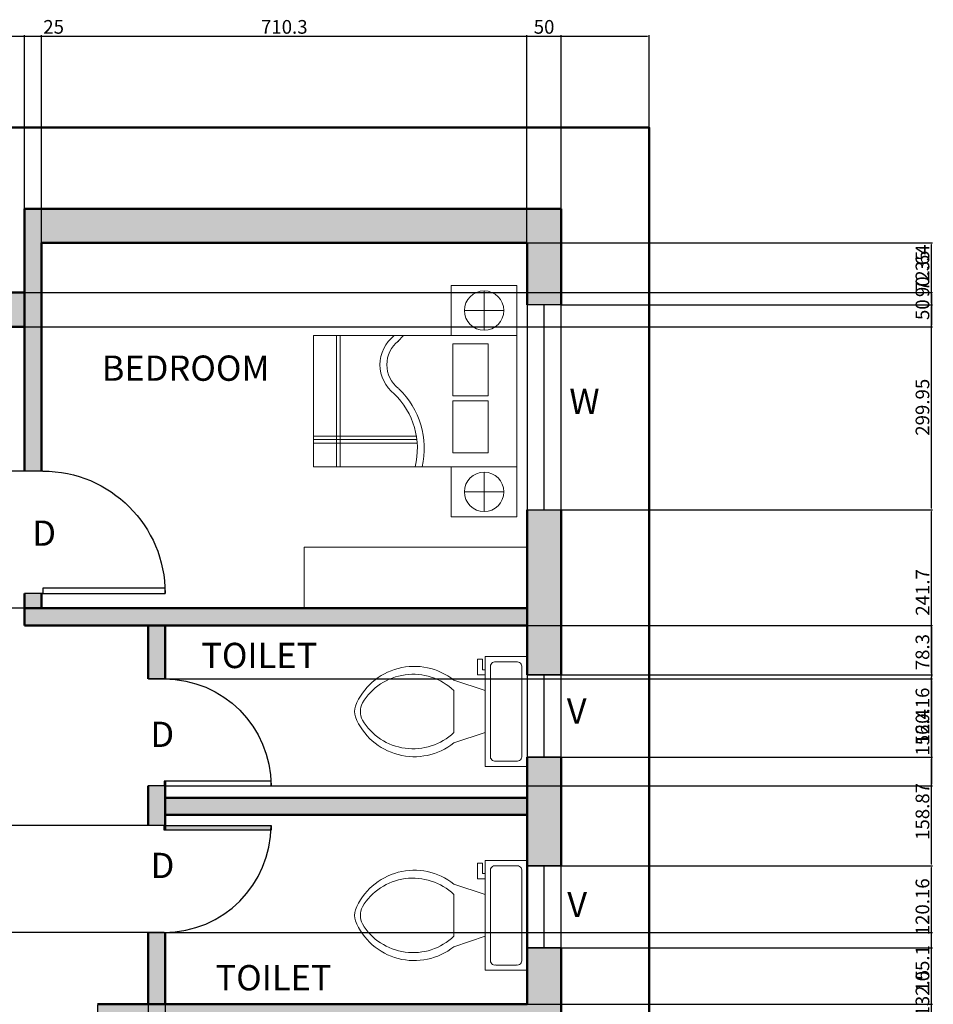
# Model space of a CAD drawing. Units: millimetres. Extents: x 1898 to 8115, y 727 to 4291.
# Tile 7 of 7: x 6778 to 8115, y 2277 to 3717. Entities that reach past the tile are written whole.
import ezdxf

# ---------------------------------------------------------------- set-up
doc = ezdxf.new("R2010")
doc.units = ezdxf.units.MM
for name, color, linetype, lineweight in [('A-ANNO-DIMS', 2, 'Continuous', 18), ('A-ANNO-TEXT', 7, 'Continuous', 25), ('A-AREA-IDEN', 3, 'Continuous', 25), ('A-DOOR', 3, 'Continuous', 25), ('A-FLOR-FIXT', 9, 'Continuous', 18), ('A-FURN', 8, 'Continuous', 18), ('A-GLAZ', 4, 'Continuous', 25), ('A-WALL', 7, 'Continuous', 50), ('A-WALL-PATT', 8, 'Continuous', 13)]:
    doc.layers.add(name, color=color, linetype=linetype, lineweight=lineweight)
doc.styles.get("Standard").update_dxf_attribs({"font": 'arial.ttf'})
doc.dimstyles.new('ISO-25', dxfattribs={"dimtxt": 20, "dimasz": 2.5, "dimexe": 1.25, "dimexo": 0.625, "dimtad": 1, "dimtxsty": 'Standard', "dimcen": 2.5, "dimadec": 0, "dimazin": 0, "dimtfac": 1, "dimtmove": 0, "dimatfit": 3, "dimfxl": 1, "dimarcsym": 0})

# ---------------------------------------------------------------- blocks, each defined once
blk = doc.blocks.new('*U43')
for p, q in [((0, 0), (0, -6)), ((40, 0), (40, -6))]:
    blk.add_line(p, q)
blk.add_lwpolyline([(0, 0), (0, 40), (1.75, 40), (1.75, 0)], close=True)
blk.add_arc((0, 0), 40, 0, 90)
blk = doc.blocks.new('*U45')
for p, q in [((9.5, -6), (9.5, -2)), ((-10, -8.5), (-8, -8.5)), ((-10, -9.5), (-10, -8.5)), ((-8, -8.5), (-8, -8)), ((-7, -8), (-7, -9.5)), ((-4, -8), (-6, -14)), ((4, -8), (6, -14)), ((-7, -9.5), (-10, -9.5)), ((4, -14), (-4, -14))]:
    blk.add_line(p, q)
blk.add_lwpolyline([(10.5, -8), (10.5, 0), (-10.5, 0), (-10.5, -8)], close=True)
for points in [[(8.5, -1), (-8.5, -1)], [(-9.5, -2), (-9.5, -6)], [(-8.5, -7), (8.5, -7)]]:
    blk.add_lwpolyline(points)
for centre, radius, start, end in [((-8.62, -1.88), 0.884, 81.8699, 188.1301), ((8.62, -1.88), 0.884, 351.8699, 98.1301), ((-8.62, -6.12), 0.884, 171.8699, 278.1301), ((8.62, -6.12), 0.884, 261.8699, 8.1301), ((3.52, -21.58), 12.17, 141.4691, 247.9714), ((4.2, -21.82), 11.33, 136.3677, 238.9468), ((-3.52, -21.58), 12.17, 292.0284, 38.5307), ((-4.2, -21.82), 11.33, 301.053, 43.6321), ((0, -27.88), 4, 245.7318, 294.2682), ((0, -29), 4, 254.8605, 285.1395)]:
    blk.add_arc(centre, radius, start, end)
blk = doc.blocks.new('*D57')
at = {"layer": 'A-ANNO-DIMS', "color": 0, "lineweight": -2, "transparency": 16777216}
for p, q in [((5348.6, 3560.4), (5348.6, 3694.5)), ((5351.1, 3693.2), (7696.3, 3693.2)), ((7698.8, 3560.4), (7698.8, 3694.5))]:
    blk.add_line(p, q, dxfattribs=at)
at = {"layer": 'A-ANNO-DIMS', "color": 0, "transparency": 16777216}
for points in [[(5351.1, 3693.7), (5351.1, 3692.8), (5348.6, 3693.2)], [(7696.3, 3693.7), (7696.3, 3692.8), (7698.8, 3693.2)]]:
    blk.add_solid(points, dxfattribs=at)
at = {"layer": 'Defpoints', "color": 0, "transparency": 16777216}
for p in [(7698.8, 3693.2), (5348.6, 3559.7), (7698.8, 3559.7)]:
    blk.add_point(p, dxfattribs=at)
at = {"layer": 'A-ANNO-DIMS', "color": 0, "transparency": 16777216, "insert": (6523.7, 3704.1), "char_height": 20, "attachment_point": 5}
blk.add_mtext('2350', dxfattribs=at)
blk = doc.blocks.new('*D58')
at = {"layer": 'A-ANNO-DIMS', "color": 0, "lineweight": -2, "transparency": 16777216}
for p, q in [((5461.6, 3441.3), (5461.6, 3694.5)), ((5464.1, 3693.2), (7567.7, 3693.2)), ((7570.2, 3441.3), (7570.2, 3694.5))]:
    blk.add_line(p, q, dxfattribs=at)
at = {"layer": 'A-ANNO-DIMS', "color": 0, "transparency": 16777216}
for points in [[(5464.1, 3693.7), (5464.1, 3692.8), (5461.6, 3693.2)], [(7567.7, 3693.7), (7567.7, 3692.8), (7570.2, 3693.2)]]:
    blk.add_solid(points, dxfattribs=at)
at = {"layer": 'Defpoints', "color": 0, "transparency": 16777216}
for p in [(7570.2, 3693.2), (5461.6, 3440.7), (7570.2, 3440.7)]:
    blk.add_point(p, dxfattribs=at)
at = {"layer": 'A-ANNO-DIMS', "color": 0, "transparency": 16777216, "insert": (6515.9, 3704.1), "char_height": 20, "attachment_point": 5}
blk.add_mtext('2108.6', dxfattribs=at)
blk = doc.blocks.new('*D66')
at = {"layer": 'A-ANNO-DIMS', "color": 0, "lineweight": -2, "transparency": 16777216}
for p, q in [((6201.7, 3318.6), (6201.7, 3694.5)), ((6204.2, 3693.2), (6782.4, 3693.2)), ((6784.9, 3318.6), (6784.9, 3694.5))]:
    blk.add_line(p, q, dxfattribs=at)
at = {"layer": 'A-ANNO-DIMS', "color": 0, "transparency": 16777216}
for points in [[(6204.2, 3693.7), (6204.2, 3692.8), (6201.7, 3693.2)], [(6782.4, 3693.7), (6782.4, 3692.8), (6784.9, 3693.2)]]:
    blk.add_solid(points, dxfattribs=at)
at = {"layer": 'Defpoints', "color": 0, "transparency": 16777216}
for p in [(6784.9, 3693.2), (6201.7, 3318), (6784.9, 3318)]:
    blk.add_point(p, dxfattribs=at)
at = {"layer": 'A-ANNO-DIMS', "color": 0, "transparency": 16777216, "insert": (6493.3, 3704.1), "char_height": 20, "attachment_point": 5}
blk.add_mtext('583.2', dxfattribs=at)
blk = doc.blocks.new('*D67')
at = {"layer": 'A-ANNO-DIMS', "color": 0, "lineweight": -2, "transparency": 16777216}
for p, q in [((6784.9, 3318.6), (6784.9, 3694.5)), ((6787.4, 3693.2), (6807.4, 3693.2)), ((6809.9, 3391.3), (6809.9, 3694.5)), ((6809.9, 3693.2), (6842.8, 3693.2))]:
    blk.add_line(p, q, dxfattribs=at)
at = {"layer": 'A-ANNO-DIMS', "color": 0, "transparency": 16777216}
for points in [[(6787.4, 3693.7), (6787.4, 3692.8), (6784.9, 3693.2)], [(6807.4, 3693.7), (6807.4, 3692.8), (6809.9, 3693.2)]]:
    blk.add_solid(points, dxfattribs=at)
at = {"layer": 'Defpoints', "color": 0, "transparency": 16777216}
for p in [(6809.9, 3693.2), (6809.9, 3390.7), (6784.9, 3318)]:
    blk.add_point(p, dxfattribs=at)
at = {"layer": 'A-ANNO-DIMS', "color": 0, "transparency": 16777216, "insert": (6827.6, 3704.1), "char_height": 20, "attachment_point": 5}
blk.add_mtext('25', dxfattribs=at)
blk = doc.blocks.new('*D68')
at = {"layer": 'A-ANNO-DIMS', "color": 0, "lineweight": -2, "transparency": 16777216}
for p, q in [((6809.9, 3391.3), (6809.9, 3694.5)), ((6812.4, 3693.2), (7517.7, 3693.2)), ((7520.2, 3391.3), (7520.2, 3694.5))]:
    blk.add_line(p, q, dxfattribs=at)
at = {"layer": 'A-ANNO-DIMS', "color": 0, "transparency": 16777216}
for points in [[(6812.4, 3693.7), (6812.4, 3692.8), (6809.9, 3693.2)], [(7517.7, 3693.7), (7517.7, 3692.8), (7520.2, 3693.2)]]:
    blk.add_solid(points, dxfattribs=at)
at = {"layer": 'Defpoints', "color": 0, "transparency": 16777216}
for p in [(7520.2, 3693.2), (6809.9, 3390.7), (7520.2, 3390.7)]:
    blk.add_point(p, dxfattribs=at)
at = {"layer": 'A-ANNO-DIMS', "color": 0, "transparency": 16777216, "insert": (7165.1, 3704.1), "char_height": 20, "attachment_point": 5}
blk.add_mtext('710.3', dxfattribs=at)
blk = doc.blocks.new('*D69')
at = {"layer": 'A-ANNO-DIMS', "color": 0, "lineweight": -2, "transparency": 16777216}
for p, q in [((7520.2, 3391.3), (7520.2, 3694.5)), ((7522.7, 3693.2), (7567.7, 3693.2)), ((7570.2, 3300.9), (7570.2, 3694.5))]:
    blk.add_line(p, q, dxfattribs=at)
at = {"layer": 'A-ANNO-DIMS', "color": 0, "transparency": 16777216}
for points in [[(7522.7, 3693.7), (7522.7, 3692.8), (7520.2, 3693.2)], [(7567.7, 3693.7), (7567.7, 3692.8), (7570.2, 3693.2)]]:
    blk.add_solid(points, dxfattribs=at)
at = {"layer": 'Defpoints', "color": 0, "transparency": 16777216}
for p in [(7570.2, 3693.2), (7520.2, 3390.7), (7570.2, 3300.3)]:
    blk.add_point(p, dxfattribs=at)
at = {"layer": 'A-ANNO-DIMS', "color": 0, "transparency": 16777216, "insert": (7545.2, 3704.1), "char_height": 20, "attachment_point": 5}
blk.add_mtext('50', dxfattribs=at)
blk = doc.blocks.new('*D94')
at = {"layer": 'A-ANNO-DIMS', "color": 0, "lineweight": -2, "transparency": 16777216}
for p, q in [((7570.8, 2359.5), (8113.5, 2359.5)), ((8112.2, 2229.5), (8112.2, 2357)), ((7570.8, 2227), (8113.5, 2227))]:
    blk.add_line(p, q, dxfattribs=at)
at = {"layer": 'A-ANNO-DIMS', "color": 0, "transparency": 16777216}
for points in [[(8111.8, 2357), (8112.7, 2357), (8112.2, 2359.5)], [(8111.8, 2229.5), (8112.7, 2229.5), (8112.2, 2227)]]:
    blk.add_solid(points, dxfattribs=at)
at = {"layer": 'Defpoints', "color": 0, "transparency": 16777216}
for p in [(7570.2, 2359.5), (8112.2, 2359.5), (7570.2, 2227)]:
    blk.add_point(p, dxfattribs=at)
at = {"layer": 'A-ANNO-DIMS', "color": 0, "transparency": 16777216, "insert": (8101.4, 2293.2), "char_height": 20, "attachment_point": 5, "rotation": 90}
blk.add_mtext('132.5', dxfattribs=at)
blk = doc.blocks.new('*D95')
at = {"layer": 'A-ANNO-DIMS', "color": 0, "lineweight": -2, "transparency": 16777216}
for p, q in [((7570.8, 2479.6), (8113.5, 2479.6)), ((8112.2, 2362), (8112.2, 2477.1)), ((7570.8, 2359.5), (8113.5, 2359.5))]:
    blk.add_line(p, q, dxfattribs=at)
at = {"layer": 'A-ANNO-DIMS', "color": 0, "transparency": 16777216}
for points in [[(8111.8, 2477.1), (8112.7, 2477.1), (8112.2, 2479.6)], [(8111.8, 2362), (8112.7, 2362), (8112.2, 2359.5)]]:
    blk.add_solid(points, dxfattribs=at)
at = {"layer": 'Defpoints', "color": 0, "transparency": 16777216}
for p in [(7570.2, 2479.6), (8112.2, 2479.6), (7570.2, 2359.5)]:
    blk.add_point(p, dxfattribs=at)
at = {"layer": 'A-ANNO-DIMS', "color": 0, "transparency": 16777216, "insert": (8101.4, 2419.6), "char_height": 20, "attachment_point": 5, "rotation": 90}
blk.add_mtext('120.16', dxfattribs=at)
blk = doc.blocks.new('*D96')
at = {"layer": 'A-ANNO-DIMS', "color": 0, "lineweight": -2, "transparency": 16777216}
for p, q in [((7570.8, 2638.5), (8113.5, 2638.5)), ((8112.2, 2482.1), (8112.2, 2636)), ((7570.8, 2479.6), (8113.5, 2479.6))]:
    blk.add_line(p, q, dxfattribs=at)
at = {"layer": 'A-ANNO-DIMS', "color": 0, "transparency": 16777216}
for points in [[(8111.8, 2636), (8112.7, 2636), (8112.2, 2638.5)], [(8111.8, 2482.1), (8112.7, 2482.1), (8112.2, 2479.6)]]:
    blk.add_solid(points, dxfattribs=at)
at = {"layer": 'Defpoints', "color": 0, "transparency": 16777216}
for p in [(7570.2, 2638.5), (8112.2, 2638.5), (7570.2, 2479.6)]:
    blk.add_point(p, dxfattribs=at)
at = {"layer": 'A-ANNO-DIMS', "color": 0, "transparency": 16777216, "insert": (8101.4, 2559.1), "char_height": 20, "attachment_point": 5, "rotation": 90}
blk.add_mtext('158.87', dxfattribs=at)
blk = doc.blocks.new('*D97')
at = {"layer": 'A-ANNO-DIMS', "color": 0, "lineweight": -2, "transparency": 16777216}
for p, q in [((7570.8, 2758.7), (8113.5, 2758.7)), ((8112.2, 2641), (8112.2, 2756.2)), ((7570.8, 2638.5), (8113.5, 2638.5))]:
    blk.add_line(p, q, dxfattribs=at)
at = {"layer": 'A-ANNO-DIMS', "color": 0, "transparency": 16777216}
for points in [[(8111.8, 2756.2), (8112.7, 2756.2), (8112.2, 2758.7)], [(8111.8, 2641), (8112.7, 2641), (8112.2, 2638.5)]]:
    blk.add_solid(points, dxfattribs=at)
at = {"layer": 'Defpoints', "color": 0, "transparency": 16777216}
for p in [(7570.2, 2758.7), (8112.2, 2758.7), (7570.2, 2638.5)]:
    blk.add_point(p, dxfattribs=at)
at = {"layer": 'A-ANNO-DIMS', "color": 0, "transparency": 16777216, "insert": (8101.4, 2698.6), "char_height": 20, "attachment_point": 5, "rotation": 90}
blk.add_mtext('120.16', dxfattribs=at)
blk = doc.blocks.new('*D98')
at = {"layer": 'A-ANNO-DIMS', "color": 0, "lineweight": -2, "transparency": 16777216}
for p, q in [((7570.8, 3000.4), (8113.5, 3000.4)), ((8112.2, 2761.2), (8112.2, 2997.9)), ((7570.8, 2758.7), (8113.5, 2758.7))]:
    blk.add_line(p, q, dxfattribs=at)
at = {"layer": 'A-ANNO-DIMS', "color": 0, "transparency": 16777216}
for points in [[(8111.8, 2997.9), (8112.7, 2997.9), (8112.2, 3000.4)], [(8111.8, 2761.2), (8112.7, 2761.2), (8112.2, 2758.7)]]:
    blk.add_solid(points, dxfattribs=at)
at = {"layer": 'Defpoints', "color": 0, "transparency": 16777216}
for p in [(7570.2, 3000.4), (8112.2, 3000.4), (7570.2, 2758.7)]:
    blk.add_point(p, dxfattribs=at)
at = {"layer": 'A-ANNO-DIMS', "color": 0, "transparency": 16777216, "insert": (8101.6, 2879.5), "char_height": 20, "attachment_point": 5, "rotation": 90}
blk.add_mtext('241.7', dxfattribs=at)
blk = doc.blocks.new('*D99')
at = {"layer": 'A-ANNO-DIMS', "color": 0, "lineweight": -2, "transparency": 16777216}
for p, q in [((7570.8, 3300.3), (8113.5, 3300.3)), ((8112.2, 3002.9), (8112.2, 3297.8)), ((7570.8, 3000.4), (8113.5, 3000.4))]:
    blk.add_line(p, q, dxfattribs=at)
at = {"layer": 'A-ANNO-DIMS', "color": 0, "transparency": 16777216}
for points in [[(8111.8, 3297.8), (8112.7, 3297.8), (8112.2, 3300.3)], [(8111.8, 3002.9), (8112.7, 3002.9), (8112.2, 3000.4)]]:
    blk.add_solid(points, dxfattribs=at)
at = {"layer": 'Defpoints', "color": 0, "transparency": 16777216}
for p in [(7570.2, 3300.3), (8112.2, 3300.3), (7570.2, 3000.4)]:
    blk.add_point(p, dxfattribs=at)
at = {"layer": 'A-ANNO-DIMS', "color": 0, "transparency": 16777216, "insert": (8101.4, 3150.3), "char_height": 20, "attachment_point": 5, "rotation": 90}
blk.add_mtext('299.95', dxfattribs=at)
blk = doc.blocks.new('*D100')
at = {"layer": 'A-ANNO-DIMS', "color": 0, "lineweight": -2, "transparency": 16777216}
for p, q in [((7520.8, 3390.7), (8113.5, 3390.7)), ((8112.2, 3302.8), (8112.2, 3388.2)), ((7570.8, 3300.3), (8113.5, 3300.3))]:
    blk.add_line(p, q, dxfattribs=at)
at = {"layer": 'A-ANNO-DIMS', "color": 0, "transparency": 16777216}
for points in [[(8111.8, 3388.2), (8112.7, 3388.2), (8112.2, 3390.7)], [(8111.8, 3302.8), (8112.7, 3302.8), (8112.2, 3300.3)]]:
    blk.add_solid(points, dxfattribs=at)
at = {"layer": 'Defpoints', "color": 0, "transparency": 16777216}
for p in [(7520.2, 3390.7), (8112.2, 3390.7), (7570.2, 3300.3)]:
    blk.add_point(p, dxfattribs=at)
at = {"layer": 'A-ANNO-DIMS', "color": 0, "transparency": 16777216, "insert": (8101.4, 3345.5), "char_height": 20, "attachment_point": 5, "rotation": 90}
blk.add_mtext('90.35', dxfattribs=at)
blk = doc.blocks.new('*D101')
at = {"layer": 'A-ANNO-DIMS', "color": 0, "lineweight": -2, "transparency": 16777216}
for p, q in [((6810.5, 3390.7), (8113.5, 3390.7)), ((8112.2, 3320.5), (8112.2, 3388.2)), ((6785.5, 3318), (8113.5, 3318))]:
    blk.add_line(p, q, dxfattribs=at)
at = {"layer": 'A-ANNO-DIMS', "color": 0, "transparency": 16777216}
for points in [[(8111.8, 3388.2), (8112.7, 3388.2), (8112.2, 3390.7)], [(8111.8, 3320.5), (8112.7, 3320.5), (8112.2, 3318)]]:
    blk.add_solid(points, dxfattribs=at)
at = {"layer": 'Defpoints', "color": 0, "transparency": 16777216}
for p in [(6809.9, 3390.7), (8112.2, 3390.7), (6784.9, 3318)]:
    blk.add_point(p, dxfattribs=at)
at = {"layer": 'A-ANNO-DIMS', "color": 0, "transparency": 16777216, "insert": (8101.4, 3354.3), "char_height": 20, "attachment_point": 5, "rotation": 90}
blk.add_mtext('72.64', dxfattribs=at)
blk = doc.blocks.new('*D102')
at = {"layer": 'A-ANNO-DIMS', "color": 0, "lineweight": -2, "transparency": 16777216}
for p, q in [((6785.5, 3318), (8113.5, 3318)), ((8112.2, 3315.5), (8112.2, 3270.5)), ((6785.5, 3268), (8113.5, 3268))]:
    blk.add_line(p, q, dxfattribs=at)
at = {"layer": 'A-ANNO-DIMS', "color": 0, "transparency": 16777216}
for points in [[(8111.8, 3315.5), (8112.7, 3315.5), (8112.2, 3318)], [(8111.8, 3270.5), (8112.7, 3270.5), (8112.2, 3268)]]:
    blk.add_solid(points, dxfattribs=at)
at = {"layer": 'Defpoints', "color": 0, "transparency": 16777216}
for p in [(6784.9, 3318), (6784.9, 3268), (8112.2, 3268)]:
    blk.add_point(p, dxfattribs=at)
at = {"layer": 'A-ANNO-DIMS', "color": 0, "transparency": 16777216, "insert": (8101.4, 3293), "char_height": 20, "attachment_point": 5, "rotation": 90}
blk.add_mtext('50', dxfattribs=at)
blk = doc.blocks.new('*D108')
at = {"layer": 'A-ANNO-DIMS', "color": 0, "lineweight": -2, "transparency": 16777216}
for p, q in [((6891.7, 2276.3), (6891.7, 1080.3)), ((6965.8, 2276.3), (6965.8, 1080.3)), ((6894.2, 1081.6), (6963.3, 1081.6))]:
    blk.add_line(p, q, dxfattribs=at)
at = {"layer": 'A-ANNO-DIMS', "color": 0, "transparency": 16777216}
for points in [[(6894.2, 1082), (6894.2, 1081.2), (6891.7, 1081.6)], [(6963.3, 1082), (6963.3, 1081.2), (6965.8, 1081.6)]]:
    blk.add_solid(points, dxfattribs=at)
at = {"layer": 'Defpoints', "color": 0, "transparency": 16777216}
for p in [(6891.7, 2277), (6965.8, 2277), (6965.8, 1081.6)]:
    blk.add_point(p, dxfattribs=at)
at = {"layer": 'A-ANNO-DIMS', "color": 0, "transparency": 16777216, "insert": (6928.8, 1092.4), "char_height": 20, "attachment_point": 5}
blk.add_mtext('74.15', dxfattribs=at)
blk = doc.blocks.new('*D109')
at = {"layer": 'A-ANNO-DIMS', "color": 0, "lineweight": -2, "transparency": 16777216}
for p, q in [((6965.8, 2276.3), (6965.8, 1080.3)), ((6990.8, 2276.3), (6990.8, 1080.3)), ((6968.3, 1081.6), (6988.3, 1081.6)), ((6990.8, 1081.6), (7023.7, 1081.6))]:
    blk.add_line(p, q, dxfattribs=at)
at = {"layer": 'A-ANNO-DIMS', "color": 0, "transparency": 16777216}
for points in [[(6968.3, 1082), (6968.3, 1081.2), (6965.8, 1081.6)], [(6988.3, 1082), (6988.3, 1081.2), (6990.8, 1081.6)]]:
    blk.add_solid(points, dxfattribs=at)
at = {"layer": 'Defpoints', "color": 0, "transparency": 16777216}
for p in [(6965.8, 2277), (6990.8, 2277), (6990.8, 1081.6)]:
    blk.add_point(p, dxfattribs=at)
at = {"layer": 'A-ANNO-DIMS', "color": 0, "transparency": 16777216, "insert": (7008.5, 1092.4), "char_height": 20, "attachment_point": 5}
blk.add_mtext('25', dxfattribs=at)
blk = doc.blocks.new('*D110')
at = {"layer": 'A-ANNO-DIMS', "color": 0, "lineweight": -2, "transparency": 16777216}
for p, q in [((6809.3, 3057), (5213.8, 3057)), ((5215.1, 2858.8), (5215.1, 3054.5)), ((6809.3, 2856.3), (5213.8, 2856.3))]:
    blk.add_line(p, q, dxfattribs=at)
at = {"layer": 'A-ANNO-DIMS', "color": 0, "transparency": 16777216}
for points in [[(5214.6, 3054.5), (5215.5, 3054.5), (5215.1, 3057)], [(5214.6, 2858.8), (5215.5, 2858.8), (5215.1, 2856.3)]]:
    blk.add_solid(points, dxfattribs=at)
at = {"layer": 'Defpoints', "color": 0, "transparency": 16777216}
for p in [(5215.1, 3057), (6809.9, 3057), (6809.9, 2856.3)]:
    blk.add_point(p, dxfattribs=at)
at = {"layer": 'A-ANNO-DIMS', "color": 0, "transparency": 16777216, "insert": (5204.2, 2956.6), "char_height": 20, "attachment_point": 5, "rotation": 90}
blk.add_mtext('200.72', dxfattribs=at)
blk = doc.blocks.new('*D111')
at = {"layer": 'A-ANNO-DIMS', "color": 0, "lineweight": -2, "transparency": 16777216}
for p, q in [((6966.5, 2831.3), (8113.5, 2831.3)), ((8112.2, 2828.8), (8112.2, 2755.5)), ((6966.5, 2753), (8113.5, 2753))]:
    blk.add_line(p, q, dxfattribs=at)
at = {"layer": 'A-ANNO-DIMS', "color": 0, "transparency": 16777216}
for points in [[(8111.8, 2828.8), (8112.7, 2828.8), (8112.2, 2831.3)], [(8111.8, 2755.5), (8112.7, 2755.5), (8112.2, 2753)]]:
    blk.add_solid(points, dxfattribs=at)
at = {"layer": 'Defpoints', "color": 0, "transparency": 16777216}
for p in [(6965.8, 2831.3), (6965.8, 2753), (8112.2, 2753)]:
    blk.add_point(p, dxfattribs=at)
at = {"layer": 'A-ANNO-DIMS', "color": 0, "transparency": 16777216, "insert": (8101.4, 2792.1), "char_height": 20, "attachment_point": 5, "rotation": 90}
blk.add_mtext('78.3', dxfattribs=at)
blk = doc.blocks.new('*D112')
at = {"layer": 'A-ANNO-DIMS', "color": 0, "lineweight": -2, "transparency": 16777216}
for p, q in [((6991.5, 2753), (8113.5, 2753)), ((8112.2, 2750.5), (8112.2, 2599.1)), ((6989.9, 2596.6), (8113.5, 2596.6))]:
    blk.add_line(p, q, dxfattribs=at)
at = {"layer": 'A-ANNO-DIMS', "color": 0, "transparency": 16777216}
for points in [[(8111.8, 2750.5), (8112.7, 2750.5), (8112.2, 2753)], [(8111.8, 2599.1), (8112.7, 2599.1), (8112.2, 2596.6)]]:
    blk.add_solid(points, dxfattribs=at)
at = {"layer": 'Defpoints', "color": 0, "transparency": 16777216}
for p in [(6990.8, 2753), (6989.3, 2596.6), (8112.2, 2596.6)]:
    blk.add_point(p, dxfattribs=at)
at = {"layer": 'A-ANNO-DIMS', "color": 0, "transparency": 16777216, "insert": (8101.4, 2674.8), "char_height": 20, "attachment_point": 5, "rotation": 90}
blk.add_mtext('156.4', dxfattribs=at)
blk = doc.blocks.new('*D113')
at = {"layer": 'A-ANNO-DIMS', "color": 0, "lineweight": -2, "transparency": 16777216}
for p, q in [((6965.2, 2538.5), (5213.8, 2538.5)), ((5215.1, 2536), (5215.1, 2384.6)), ((6965.2, 2382.1), (5213.8, 2382.1))]:
    blk.add_line(p, q, dxfattribs=at)
at = {"layer": 'A-ANNO-DIMS', "color": 0, "transparency": 16777216}
for points in [[(5214.6, 2536), (5215.5, 2536), (5215.1, 2538.5)], [(5214.6, 2384.6), (5215.5, 2384.6), (5215.1, 2382.1)]]:
    blk.add_solid(points, dxfattribs=at)
at = {"layer": 'Defpoints', "color": 0, "transparency": 16777216}
for p in [(6965.8, 2538.5), (5215.1, 2382.1), (6965.8, 2382.1)]:
    blk.add_point(p, dxfattribs=at)
at = {"layer": 'A-ANNO-DIMS', "color": 0, "transparency": 16777216, "insert": (5204.2, 2460.3), "char_height": 20, "attachment_point": 5, "rotation": 90}
blk.add_mtext('156.42', dxfattribs=at)
blk = doc.blocks.new('*D114')
at = {"layer": 'A-ANNO-DIMS', "color": 0, "lineweight": -2, "transparency": 16777216}
for p, q in [((6966.5, 2382.1), (8113.5, 2382.1)), ((8112.2, 2279.5), (8112.2, 2379.6)), ((6966.5, 2277), (8113.5, 2277))]:
    blk.add_line(p, q, dxfattribs=at)
at = {"layer": 'A-ANNO-DIMS', "color": 0, "transparency": 16777216}
for points in [[(8111.8, 2379.6), (8112.7, 2379.6), (8112.2, 2382.1)], [(8111.8, 2279.5), (8112.7, 2279.5), (8112.2, 2277)]]:
    blk.add_solid(points, dxfattribs=at)
at = {"layer": 'Defpoints', "color": 0, "transparency": 16777216}
for p in [(6965.8, 2382.1), (8112.2, 2382.1), (6965.8, 2277)]:
    blk.add_point(p, dxfattribs=at)
at = {"layer": 'A-ANNO-DIMS', "color": 0, "transparency": 16777216, "insert": (8101.4, 2329.5), "char_height": 20, "attachment_point": 5, "rotation": 90}
blk.add_mtext('105.1', dxfattribs=at)

msp = doc.modelspace()

# ---------------------------------------------------------------- hatches: boundary and pattern name
at = {"layer": 'A-WALL-PATT'}
h = msp.add_hatch(color=256, dxfattribs=at)
h.dxf.hatch_style = 1
h.paths.add_polyline_path([(6201.726, 3440.661), (5461.585, 3440.661), (5461.585, 3265.221), (5511.585, 3265.221), (5511.585, 3390.661), (6176.726, 3390.661), (6176.726, 2856.284), (6201.726, 2856.284)])
h.paths.add_polyline_path([(6784.895, 3318.017), (6201.726, 3318.017), (6201.726, 3268.017), (6784.895, 3268.017)])
h.paths.add_polyline_path([(7570.217, 3440.661), (6784.895, 3440.661), (6784.895, 3057.009), (6809.895, 3057.009), (6809.895, 3390.661), (7520.217, 3390.661), (7520.217, 3300.311), (7570.217, 3300.311)])
h.paths.add_polyline_path([(7570.217, 3000.359), (7520.217, 3000.359), (7520.217, 2758.681), (7570.217, 2758.681)])
h.paths.add_polyline_path([(7520.217, 2856.284), (7194.283, 2856.284), (6784.895, 2856.284), (6784.895, 2831.284), (7520.217, 2831.284)])
h.paths.add_polyline_path([(6809.895, 2878.069), (6784.895, 2878.069), (6784.895, 2856.284), (6809.895, 2856.284)])
h.paths.add_polyline_path([(6201.726, 2856.284), (6176.726, 2856.284), (6161.551, 2856.284), (6161.551, 2831.284), (6201.726, 2831.284)])
h.paths.add_polyline_path([(5905.861, 2856.284), (5511.585, 2856.284), (5511.585, 2831.284), (5905.861, 2831.284)])
h.paths.add_polyline_path([(5511.585, 2965.269), (5461.585, 2965.269), (5461.585, 2698.678), (5511.585, 2698.678)])
h.paths.add_polyline_path([(5511.585, 2398.725), (5461.585, 2398.725), (5461.585, 2088.028), (5511.585, 2088.028)])
h.paths.add_polyline_path([(5989.6, 2238.621), (5989.6, 2276.975), (5511.585, 2276.975), (5511.585, 2226.975), (5989.865, 2226.975, -0.01139164)])
h.paths.add_polyline_path([(6636.013, 2276.975), (6245.29, 2276.975), (6245.29, 2238.621), (6245.29, 2226.975), (6636.013, 2226.975), (6636.013, 2238.621)])
h.paths.add_polyline_path([(7570.217, 2359.481), (7520.217, 2359.481), (7520.217, 2326.802), (7520.217, 2276.975), (6891.704, 2276.975), (6891.704, 2238.621, -0.01139164), (6891.439, 2226.975), (7570.217, 2226.975)])
h.paths.add_polyline_path([(7145.586, 2531.644), (6989.313, 2531.644), (6989.313, 2538.488), (7145.735, 2538.488), (7145.735, 2531.644), (7145.586, 2531.644, -0.39860379), (6990.849, 2382.073), (6990.849, 2276.975), (6965.849, 2276.975), (6965.849, 2382.065), (6989.313, 2382.065, 0.40145271)])
h.paths.add_polyline_path([(6990.849, 2596.561), (6989.313, 2596.561), (6965.849, 2596.561), (6965.849, 2538.488), (6990.849, 2538.488)])
h.paths.add_polyline_path([(6990.849, 2831.284), (6965.849, 2831.284), (6965.849, 2752.984), (6990.849, 2752.984)])
h.paths.add_polyline_path([(7570.217, 2638.517), (7520.217, 2638.517), (7520.217, 2625.002), (7520.217, 2479.644), (7570.217, 2479.644)])
h.paths.add_polyline_path([(7520.217, 2579.13), (6990.849, 2579.13), (6990.849, 2554.13), (7520.217, 2554.13)])

# ---------------------------------------------------------------- linework, layer by layer
at = {"layer": 'A-FURN'}
for p, q in [((7457.414, 3262.89), (7457.414, 3320.499)), ((7486.219, 3291.695), (7428.61, 3291.695)), ((7241.696, 3063.119), (7241.696, 3255.036)), ((7246.696, 3063.119), (7246.696, 3255.036)), ((7331.427, 3246.671), (7339.669, 3255.036)), ((7359.058, 3107.895), (7207.596, 3107.895)), ((7359.058, 3102.895), (7207.596, 3102.895)), ((7359.058, 3097.895), (7207.596, 3097.895)), ((7457.414, 2997.657), (7457.414, 3055.266)), ((7486.219, 3026.461), (7428.61, 3026.461))]:
    msp.add_line(p, q, dxfattribs=at)
for points in [[(7505.435, 3255.036), (7409.393, 3255.036), (7409.393, 3328.353), (7505.435, 3328.353)], [(7505.435, 3255.036), (7207.596, 3255.036), (7207.596, 3063.119), (7505.435, 3063.119)], [(7463.586, 3167.185), (7411.519, 3167.185), (7411.519, 3243.164), (7463.586, 3243.164)], [(7463.586, 3083.676), (7411.519, 3083.676), (7411.519, 3159.655), (7463.586, 3159.655)], [(7505.435, 2989.803), (7409.393, 2989.803), (7409.393, 3063.119), (7505.435, 3063.119)], [(7194.283, 2856.284), (7520.217, 2856.284), (7520.217, 2945.821), (7194.283, 2945.821)]]:
    msp.add_lwpolyline(points, close=True, dxfattribs=at)
for centre in [(7457.414, 3291.695), (7457.414, 3026.461)]:
    msp.add_circle(centre, 28.804, dxfattribs=at)
for centre, radius, start, end in [((7359.1, 3212.48), 53.987, 127.974461, 232.025539), ((7359.1, 3212.48), 43.987, 127.974461, 232.025539), ((7248.669, 3089.981), 111.142, 346.014043, 45.994834), ((7248.669, 3089.981), 121.142, 347.189123, 45.994834)]:
    msp.add_arc(centre, radius, start, end, dxfattribs=at)
at = {"layer": 'A-GLAZ'}
for p, q in [((7545.217, 3000.359), (7545.217, 3300.311)), ((7545.217, 2638.517), (7545.217, 2758.681)), ((7545.217, 2359.481), (7545.217, 2479.644))]:
    msp.add_line(p, q, dxfattribs=at)
for points in [[(7570.217, 3300.311), (7520.217, 3300.311)], [(7520.217, 3000.359), (7570.217, 3000.359)], [(7520.217, 2758.681), (7570.217, 2758.681)], [(7570.217, 2638.517), (7520.217, 2638.517)], [(7570.217, 2359.481), (7520.217, 2359.481), (7520.217, 2479.644), (7570.217, 2479.644)]]:
    msp.add_lwpolyline(points, dxfattribs=at)
for points in [[(7520.217, 3000.359), (7570.217, 3000.359), (7570.217, 3300.311), (7520.217, 3300.311)], [(7520.217, 2638.517), (7570.217, 2638.517), (7570.217, 2758.681), (7520.217, 2758.681)], [(7520.217, 2359.481), (7570.217, 2359.481), (7570.217, 2479.644), (7520.217, 2479.644)]]:
    msp.add_lwpolyline(points, close=True, dxfattribs=at)
at = {"layer": 'A-WALL'}
for p, q in [((6784.895, 3440.661), (7570.217, 3440.661)), ((6784.895, 3440.661), (6784.895, 3057.009)), ((7570.217, 3440.661), (7570.217, 3300.311)), ((6809.895, 3390.661), (6809.895, 3057.009)), ((6809.895, 3390.661), (7520.217, 3390.661)), ((7520.217, 3390.661), (7520.217, 3300.311)), ((6201.726, 3318.017), (6784.895, 3318.017)), ((6201.726, 3268.017), (6784.895, 3268.017)), ((7520.217, 3000.359), (7520.217, 2758.681)), ((7570.217, 3000.359), (7570.217, 2758.681)), ((6784.895, 2878.069), (6784.895, 2856.284)), ((6809.895, 2878.069), (6809.895, 2856.284)), ((6784.895, 2856.284), (6784.895, 2831.284)), ((6784.895, 2856.284), (7520.217, 2856.284)), ((6784.895, 2831.284), (7520.217, 2831.284)), ((6965.849, 2831.284), (6965.849, 2752.984)), ((6990.849, 2831.284), (6990.849, 2752.976)), ((7520.217, 2638.517), (7520.217, 2276.975)), ((7570.217, 2638.517), (7570.217, 2479.644)), ((6965.849, 2596.561), (6965.849, 2538.488)), ((6990.849, 2603.405), (6990.849, 2531.644)), ((6990.849, 2579.13), (7520.217, 2579.13)), ((6990.849, 2554.13), (7520.217, 2554.13)), ((6965.849, 2382.065), (6965.849, 2276.975)), ((6990.849, 2382.073), (6990.849, 2276.975)), ((7570.217, 2359.481), (7570.217, 2226.975)), ((6891.704, 2276.975), (7520.217, 2276.975))]:
    msp.add_line(p, q, dxfattribs=at)
msp.add_lwpolyline([(5348.551, 3559.737), (7698.767, 3559.737), (7698.767, 1496.544), (5348.551, 1496.544)], close=True, dxfattribs=at)

# ---------------------------------------------------------------- block references
at = {"layer": 'A-DOOR', "rotation": 270}
for p, xscale, yscale, zscale in [((6811.736, 2878.069), -4.473499010525142, 4.473499010525142, 4.473499010525142), ((6989.313, 2596.561), -3.91056328234218, 3.91056328234218, 3.91056328234218), ((6989.313, 2538.488), 3.91056328234218, 3.91056328234218, 3.91056328234218)]:
    msp.add_blockref('*U43', p, dxfattribs=dict(at, xscale=xscale, yscale=yscale, zscale=zscale))
at = {"layer": 'A-FLOR-FIXT', "xscale": 7.642125996577618, "yscale": 7.642125996577618, "zscale": 7.642125996577618, "rotation": 270}
for p in [(7520.217, 2705.244), (7520.217, 2407.044)]:
    msp.add_blockref('*U45', p, dxfattribs=at)

# ---------------------------------------------------------------- texts
at = {"layer": 'A-ANNO-TEXT', "char_height": 36.981, "attachment_point": 1}
for s, insert in [('W', (7582.139, 3177.543)), ('D', (6796.387, 2984.607)), ('V', (7578.419, 2724.618)), ('D', (6969.208, 2690.37)), ('D', (6969.561, 2498.593)), ('V', (7579.077, 2441.462))]:
    msp.add_mtext_dynamic_manual_height_columns(s, width=5503.90807, gutter_width=184.907, heights=[0], dxfattribs=dict(at, insert=insert))
at = {"layer": 'A-AREA-IDEN', "char_height": 36.9814, "attachment_point": 1}
for s, insert in [('BEDROOM', (6898.013, 3225.968)), ('TOILET', (7043.585, 2805.724)), ('TOILET', (7064.458, 2334.362))]:
    msp.add_mtext_dynamic_manual_height_columns(s, width=5503.90807, gutter_width=184.907, heights=[0], dxfattribs=dict(at, insert=insert))

# ---------------------------------------------------------------- dimensions: what is measured, and where the dimension line sits
at = {"layer": 'A-ANNO-DIMS'}
for base, p1, p2, override, picture, middle in [((7698.767, 3693.237), (5348.551, 3559.737), (7698.767, 3559.737), {"dimdec": 0, "dimlfac": 1, "dimrnd": 0, "dimzin": 0, "dimdsep": 46, "dimlunit": 2}, '*D57', (6523.659, 3704.08)), ((7570.217, 3693.237), (5461.585, 3440.661), (7570.217, 3440.661), {"dimdec": 1, "dimlfac": 1, "dimrnd": 0, "dimzin": 0, "dimdsep": 46, "dimlunit": 2}, '*D58', (6515.901, 3704.073)), ((6784.895, 3693.237), (6201.726, 3318.017), (6784.895, 3318.017), {"dimdec": 1, "dimlfac": 1, "dimrnd": 0, "dimzin": 0, "dimdsep": 46, "dimlunit": 2}, '*D66', (6493.31, 3704.08)), ((6809.895, 3693.237), (6784.895, 3318.017), (6809.895, 3390.661), {"dimdec": 0, "dimlfac": 1, "dimrnd": 0, "dimzin": 0, "dimdsep": 46, "dimlunit": 2}, '*D67', (6827.59, 3704.073)), ((7520.217, 3693.237), (6809.895, 3390.661), (7520.217, 3390.661), {"dimdec": 1, "dimlfac": 1, "dimrnd": 0, "dimzin": 0, "dimdsep": 46, "dimlunit": 2}, '*D68', (7165.056, 3704.08)), ((7570.217, 3693.237), (7520.217, 3390.661), (7570.217, 3300.311), {"dimdec": 0, "dimlfac": 1, "dimrnd": 0, "dimzin": 0, "dimdsep": 46, "dimlunit": 2}, '*D69', (7545.217, 3704.073)), ((6965.8494, 1081.5935), (6891.704, 2276.9748), (6965.8494, 2276.9748), {"dimdec": 2, "dimlfac": 1, "dimrnd": 0, "dimzin": 0, "dimdsep": 46, "dimlunit": 2}, '*D108', (6928.7767, 1092.43)), ((6990.849, 1081.594), (6965.849, 2276.975), (6990.849, 2276.975), {"dimdec": 0, "dimlfac": 1, "dimrnd": 0, "dimzin": 0, "dimdsep": 46, "dimlunit": 2}, '*D109', (7008.545, 1092.43))]:
    dim = msp.add_linear_dim(base=base, p1=p1, p2=p2, dimstyle='ISO-25', override=override, dxfattribs=at)
    dim.commit()
    dim.dimension.update_dxf_attribs({"geometry": picture, "text_midpoint": middle})
for base, p1, p2, override, picture, middle in [((8112.244, 3390.661), (6784.895, 3318.017), (6809.895, 3390.661), {"dimdec": 2, "dimlfac": 1, "dimrnd": 0, "dimzin": 0, "dimdsep": 46, "dimlunit": 2}, '*D101', (8101.408, 3354.339)), ((8112.244, 3390.661), (7570.217, 3300.311), (7520.217, 3390.661), {"dimdec": 2, "dimlfac": 1, "dimrnd": 0, "dimzin": 0, "dimdsep": 46, "dimlunit": 2}, '*D100', (8101.401, 3345.486)), ((8112.244, 3268.017), (6784.895, 3318.017), (6784.895, 3268.017), {"dimdec": 0, "dimlfac": 1, "dimrnd": 0, "dimzin": 0, "dimdsep": 46, "dimlunit": 2}, '*D102', (8101.408, 3293.017)), ((8112.244, 3300.311), (7570.217, 3000.359), (7570.217, 3300.311), {"dimdec": 2, "dimlfac": 1, "dimrnd": 0, "dimzin": 0, "dimdsep": 46, "dimlunit": 2}, '*D99', (8101.408, 3150.335)), ((5215.0506, 3057.0088), (6809.8949, 2856.2845), (6809.8949, 3057.0088), {"dimdec": 2, "dimlfac": 1, "dimrnd": 0, "dimzin": 0, "dimdsep": 46, "dimlunit": 2}, '*D110', (5204.2141, 2956.6467)), ((8112.244, 3000.359), (7570.217, 2758.681), (7570.217, 3000.359), {"dimdec": 1, "dimlfac": 1, "dimrnd": 0, "dimzin": 0, "dimdsep": 46, "dimlunit": 2}, '*D98', (8101.578, 2879.52)), ((8112.244, 2752.984), (6965.849, 2831.284), (6965.849, 2752.984), {"dimdec": 1, "dimlfac": 1, "dimrnd": 0, "dimzin": 0, "dimdsep": 46, "dimlunit": 2}, '*D111', (8101.401, 2792.134)), ((8112.244, 2596.561), (6990.849, 2752.976), (6989.313, 2596.561), {"dimdec": 1, "dimlfac": 1, "dimrnd": 0, "dimzin": 0, "dimdsep": 46, "dimlunit": 2}, '*D112', (8101.408, 2674.769)), ((8112.244, 2758.681), (7570.217, 2638.517), (7570.217, 2758.681), {"dimdec": 2, "dimlfac": 1, "dimrnd": 0, "dimzin": 0, "dimdsep": 46, "dimlunit": 2}, '*D97', (8101.408, 2698.599)), ((8112.244, 2638.517), (7570.217, 2479.644), (7570.217, 2638.517), {"dimdec": 2, "dimlfac": 1, "dimrnd": 0, "dimzin": 0, "dimdsep": 46, "dimlunit": 2}, '*D96', (8101.408, 2559.081)), ((5215.051, 2382.065), (6965.849, 2538.488), (6965.849, 2382.065), {"dimdec": 2, "dimlfac": 1, "dimrnd": 0, "dimzin": 0, "dimdsep": 46, "dimlunit": 2}, '*D113', (5204.214, 2460.277)), ((8112.244, 2479.644), (7570.217, 2359.481), (7570.217, 2479.644), {"dimdec": 2, "dimlfac": 1, "dimrnd": 0, "dimzin": 0, "dimdsep": 46, "dimlunit": 2}, '*D95', (8101.408, 2419.563)), ((8112.244, 2382.065), (6965.849, 2276.975), (6965.849, 2382.065), {"dimdec": 1, "dimlfac": 1, "dimrnd": 0, "dimzin": 0, "dimdsep": 46, "dimlunit": 2}, '*D114', (8101.408, 2329.52)), ((8112.244, 2359.481), (7570.217, 2226.975), (7570.217, 2359.481), {"dimdec": 1, "dimlfac": 1, "dimrnd": 0, "dimzin": 0, "dimdsep": 46, "dimlunit": 2}, '*D94', (8101.401, 2293.228))]:
    dim = msp.add_linear_dim(base=base, p1=p1, p2=p2, angle=90, dimstyle='ISO-25', override=override, dxfattribs=at)
    dim.commit()
    dim.dimension.update_dxf_attribs({"geometry": picture, "text_midpoint": middle})

doc.saveas('drawing.dxf')
